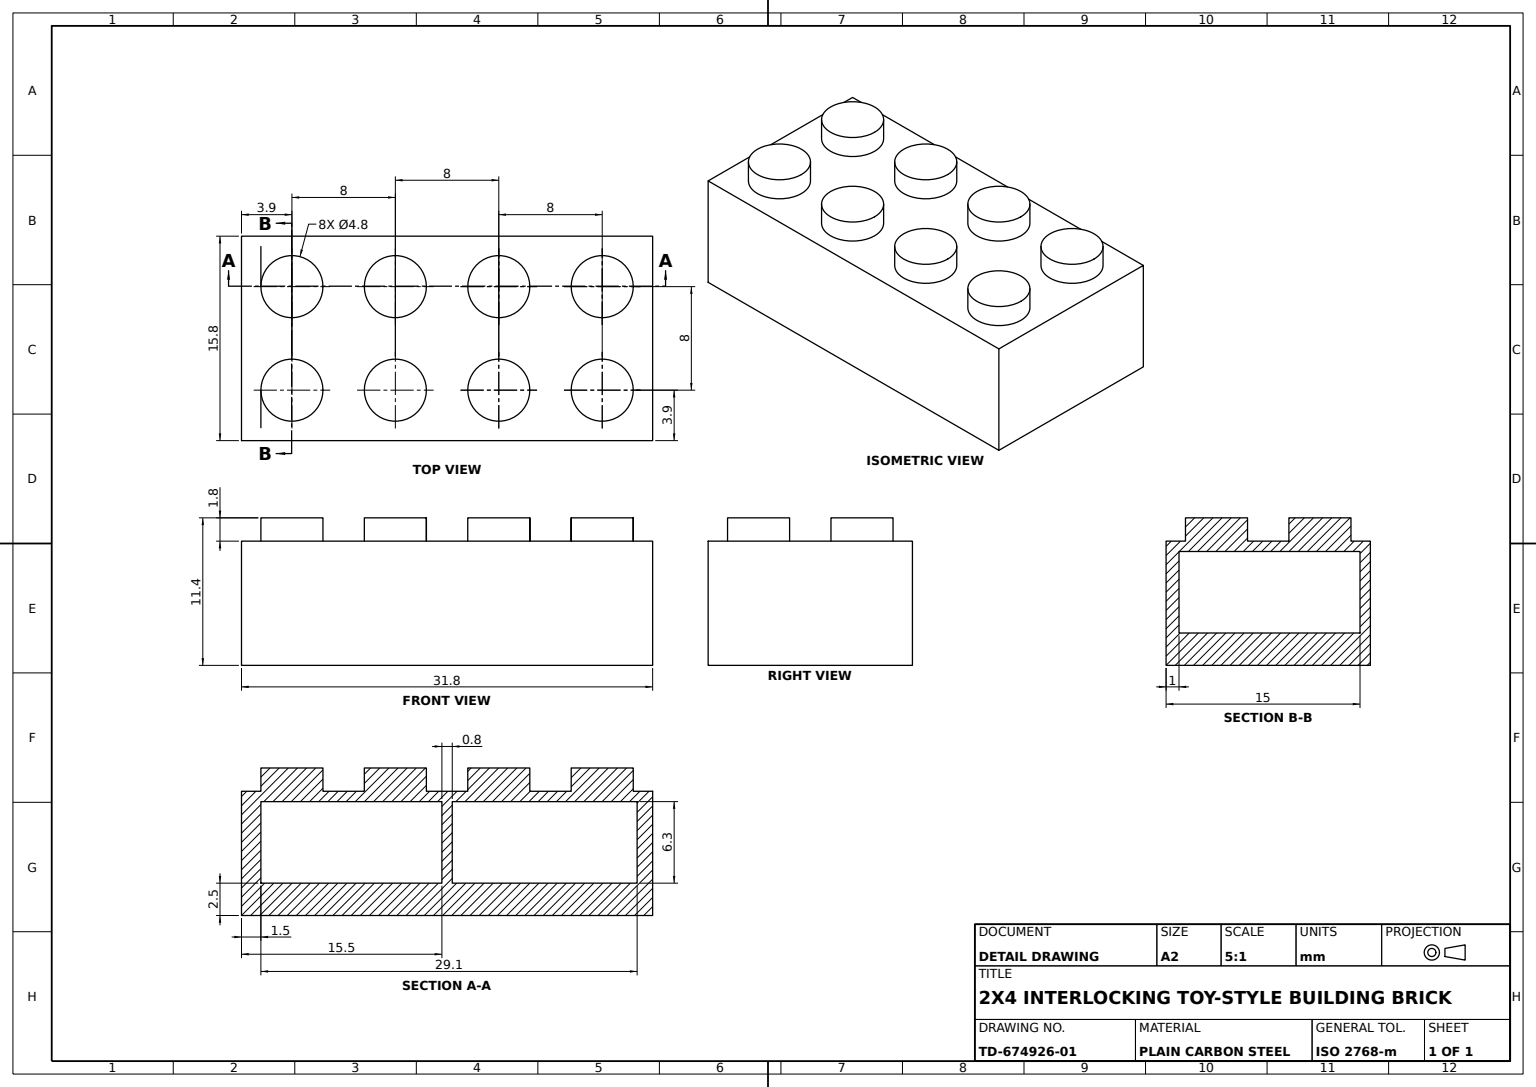
SolidWorks part; units mm, degrees
material "Plain Carbon Steel"
ref_plane "Front Plane" through (0, 0, 0) normal (0, 0, 1) x (1, 0, 0)
ref_plane "Top Plane" through (0, 0, 0) normal (0, 1, 0) x (1, 0, 0)
ref_plane "Right Plane" through (0, 0, 0) normal (1, 0, 0) x (0, 0, -1)
sketch "Brick Outline Sketch" plane through (0, 0, 0) normal (0, 0, 1) x (1, 0, 0)
  line L0 (0, 0) -> (0, 15.8)
  line L1 (0, 15.8) -> (31.8, 15.8)
  line L2 (31.8, 15.8) -> (31.8, 0)
  line L3 (31.8, 0) -> (0, 0)
  dimension "D1" = 15.8
  dimension "D2" = 31.8
  dimension "D3" = 15.8
extrude "Brick Body 9.6" add sketch "Brick Outline Sketch" along normal blind 9.6
sketch "Stud Circles Sketch" plane through (0, 0, 9.6) normal (0, 0, 1) x (1, 0, 0)
  line L0 (0, 15.8) -> (0, 0) construction
  line L1 (31.8, 15.8) -> (0, 15.8) construction
  line L2 (0, 0) -> (31.8, 0) construction
  circle A0 centre (3.9, 11.9) radius 2.4
  circle A1 centre (3.9, 3.9) radius 2.4
  circle A2 centre (11.9, 11.9) radius 2.4
  circle A3 centre (19.9, 11.9) radius 2.4
  circle A4 centre (27.9, 11.9) radius 2.4
  circle A5 centre (11.9, 3.9) radius 2.4
  circle A6 centre (19.9, 3.9) radius 2.4
  circle A7 centre (27.9, 3.9) radius 2.4
  dimension "D1" = 4.8
  dimension "D2" = 4.8
  dimension "D3" = 4.8
  dimension "D4" = 4.8
  dimension "D5" = 4.8
  dimension "D6" = 4.8
  dimension "D7" = 4.8
  dimension "D8" = 4.8
  dimension "D9" = 3.9
  dimension "D10" = 3.9
  dimension "D11" = 3.9
  dimension "D12" = 3.9
  dimension "D13" = 3.9
  dimension "D14" = 8
  dimension "D15" = 3.9
  dimension "D16" = 8
  dimension "D17" = 3.9
  dimension "D18" = 8
  dimension "D19" = 3.9
  dimension "D20" = 8
  dimension "D21" = 3.9
  dimension "D22" = 8
  dimension "D23" = 3.9
  dimension "D24" = 8
extrude "Studs 8xØ4.8" add sketch "Stud Circles Sketch" along normal blind 1.8
sketch "Underside Cut Sketch" plane through (0, 0, 0) normal (0, -1, 0) x (1, 0, 0)
  line L0 (31.8, 9.6) -> (31.8, 0) construction
  line L1 (0, 0) -> (31.8, 0) construction
  line L2 (1.5, 8.8) -> (1.5, 2.5)
  line L3 (1.5, 2.5) -> (30.6, 2.5)
  line L6 (30.6, 2.5) -> (30.6, 8.8)
  line L7 (30.6, 8.8) -> (1.5, 8.8)
  line L10 (15.5, 8.8) -> (15.5, 2.5)
  line L11 (15.5, 2.5) -> (16.3, 2.5)
  line L12 (16.3, 2.5) -> (16.3, 8.8)
  line L13 (15.5, 8.8) -> (16.3, 8.8)
  dimension "D1" = 1.2
  dimension "D2" = 6.3
  dimension "D3" = 15.5
  dimension "D4" = 29.1
  dimension "D5" = 2.5
  dimension "D6" = 0.8
extrude "Underside Cut" cut sketch "Underside Cut Sketch" against normal blind 15 contours L10 L7 L2 L3 | L12 L3 L6 L7
sketch "Underside Boss Sketch" plane through (0, 0, 0) normal (0, -1, 0) x (1, 0, 0)
  line L0 (1.5, 8.8) -> (15.5, 8.8)
  line L1 (15.5, 8.8) -> (15.5, 2.5)
  line L2 (15.5, 2.5) -> (1.5, 2.5)
  line L3 (1.5, 2.5) -> (1.5, 8.8)
  line L4 (16.3, 8.8) -> (30.6, 8.8)
  line L5 (30.6, 8.8) -> (30.6, 2.5)
  line L6 (30.6, 2.5) -> (16.3, 2.5)
  line L7 (16.3, 2.5) -> (16.3, 8.8)
extrude "Underside Boss 1mm" add sketch "Underside Boss Sketch" against normal blind 1
